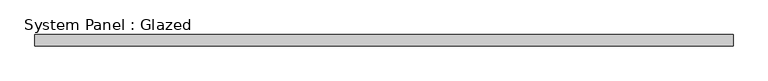
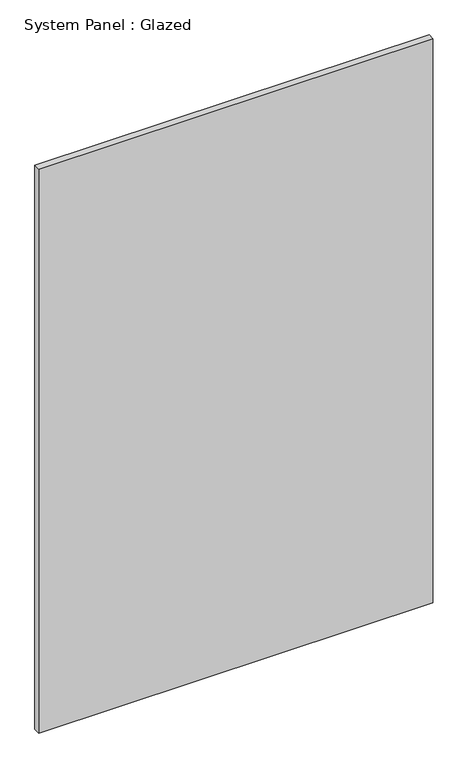
"""IFC4 building model written with IfcOpenShell, lengths in millimetres: plate geometry, System Panel : Glazed."""

from ifc_helpers import new_model, si_unit, origin, origin_with_axes, place, context, project, spatial, polyline, outline, extrude, source, transform, mapped, element, save


def system_panel_glazed_3bb4e025(model_context):
    return source(origin(), model_context, "Body", "SweptSolid", [
        extrude(outline(polyline([(787.4, 19.05), (-787.4, 19.05), (-787.4, 44.45), (787.4, 44.45), (787.4, 19.05)])), origin_with_axes(), (0.0, 0.0, 1.0), 2381.9724322),
    ])


if __name__ == "__main__":
    model = new_model("IFC4")
    model_context = context("Model", 3, world=origin())
    ifc_project = project(units=[si_unit("LENGTHUNIT", "METRE", prefix="MILLI")], contexts=[model_context])
    site = spatial("IfcSite", under=ifc_project)
    building = spatial("IfcBuilding", under=site)
    placement = place(None, origin())
    system_panel_glazed_shape = system_panel_glazed_3bb4e025(model_context)
    element("IfcPlate", 1, ObjectType="System Panel : Glazed", at=placement, inside=building, context=model_context, shape_type="MappedRepresentation", body=[
        mapped(system_panel_glazed_shape, transform((0.0, 0.0, 0.0), x_axis=(1.0, 0.0, 0.0), y_axis=(0.0, 1.0, 0.0), z_axis=(0.0, 0.0, 1.0))),
    ])
    save(model, "model.ifc")

# Revit data of these elements
# Type "System Panel : Glazed"
#   Construction Type Id = "GSP4R"
#   Analytic Construction = "1/8 in Pilkington single glazing"
#   Visual Light Transmittance = 0.9
#   Solar Heat Gain Coefficient = 0.86
#   Heat Transfer Coefficient (U) = 1.18115 BTU/(h·ft²·°F)
# Element 1 (IfcPlate, "System Panel : Glazed")
#   Materials on its faces: "Glass"
# Materials
#   "Glass": class "Glass", colour RGB 0 128 192, transparency 0.75, Description = "Soda Lime Glass", Cost = 0
